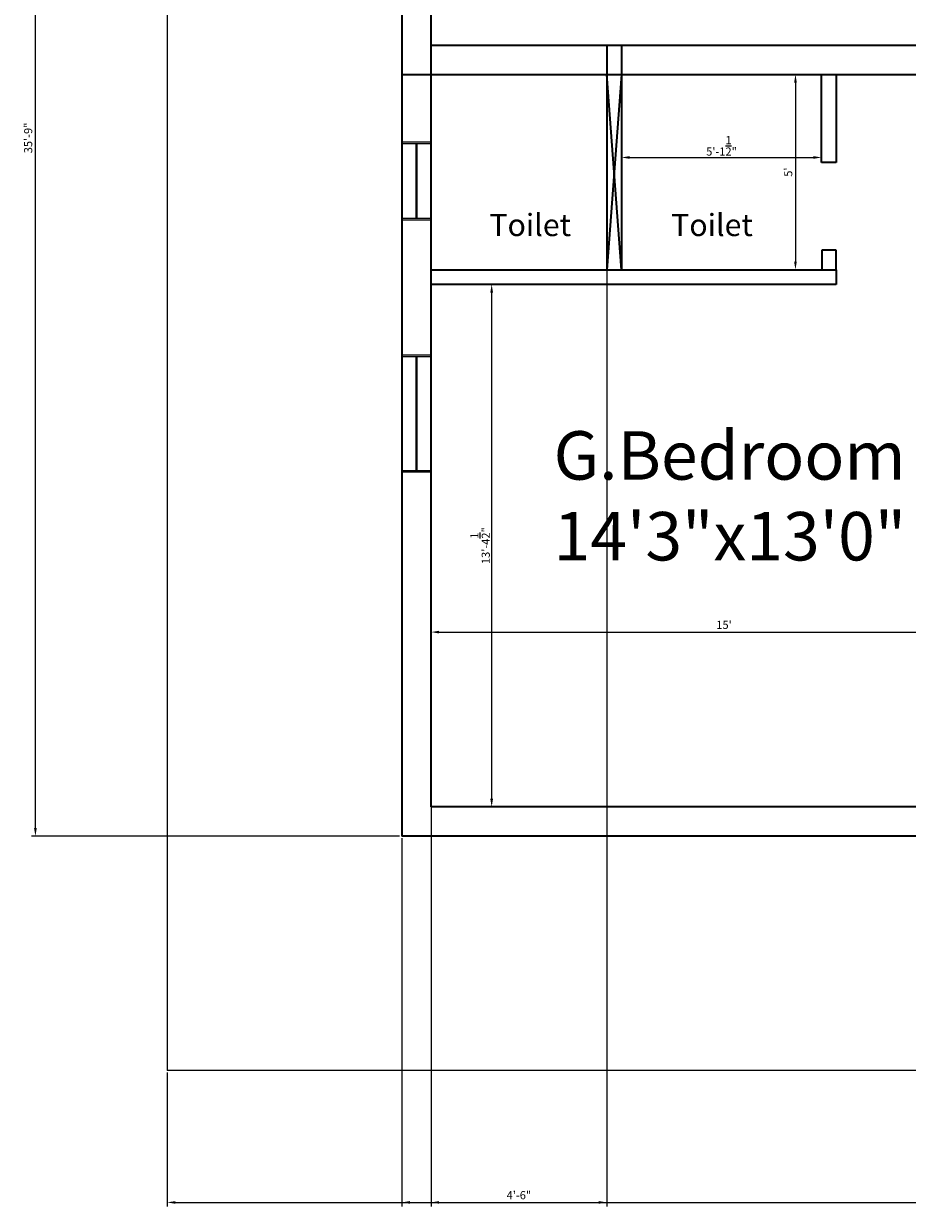
# Model space of a CAD drawing. Units: inches. Extents: x 250205121 to 250208111, y 89832590 to 89833271.
# Tile 5 of 14: x 250206174 to 250206445, y 89832600 to 89832964. Entities that reach past the tile are written whole.
import ezdxf

# ---------------------------------------------------------------- set-up
doc = ezdxf.new("R2010")
doc.units = ezdxf.units.IN
for name, color, linetype, lineweight in [('A-AREA-IDEN', 4, 'Continuous', 18), ('A-WALL', 7, 'Continuous', 35), ('C-PROP', 8, 'Continuous', 25), ('dimensions', 2, 'Continuous', 18), ('window', 4, 'Continuous', 18)]:
    doc.layers.add(name, color=color, linetype=linetype, lineweight=lineweight)
doc.styles.get("Standard").update_dxf_attribs({"font": 'arial.ttf'})
doc.dimstyles.new('ISO-25', dxfattribs={"dimtxt": 2.5, "dimasz": 2.5, "dimexe": 1.25, "dimexo": 0.625, "dimtad": 1, "dimlunit": 4, "dimtxsty": 'Standard', "dimcen": 2.5, "dimadec": 0, "dimazin": 0, "dimtfac": 1, "dimtmove": 0, "dimatfit": 3, "dimfxl": 1, "dimarcsym": 0})

# ---------------------------------------------------------------- blocks, each defined once
blk = doc.blocks.new('*D12')
at = {"layer": 'Defpoints', "color": 0, "transparency": 16777216}
for p in [(250206357.69, 89832922.83), (250206419.16, 89832922.83), (250206419.16, 89832922.83)]:
    blk.add_point(p, dxfattribs=at)
at = {"layer": 'dimensions', "color": 0, "lineweight": -2, "transparency": 16777216}
for p, q in [((250206357.69, 89832923.45), (250206357.69, 89832924.08)), ((250206360.19, 89832922.83), (250206416.66, 89832922.83)), ((250206419.16, 89832923.45), (250206419.16, 89832924.08))]:
    blk.add_line(p, q, dxfattribs=at)
at = {"layer": 'dimensions', "color": 0, "transparency": 16777216}
for points in [[(250206360.19, 89832923.24), (250206360.19, 89832922.41), (250206357.69, 89832922.83)], [(250206416.66, 89832923.24), (250206416.66, 89832922.41), (250206419.16, 89832922.83)]]:
    blk.add_solid(points, dxfattribs=at)
at = {"layer": 'dimensions', "color": 0, "transparency": 16777216, "insert": (250206388.43, 89832926.4), "char_height": 2.5, "attachment_point": 5}
blk.add_mtext('5\'-1{\\H1x;\\S1/2;}"', dxfattribs=at)
blk = doc.blocks.new('*D13')
at = {"layer": 'Defpoints', "color": 0, "transparency": 16777216}
for p in [(250206401.38, 89832948.33), (250206401.38, 89832888.33), (250206411.13, 89832888.33)]:
    blk.add_point(p, dxfattribs=at)
at = {"layer": 'dimensions', "color": 0, "lineweight": -2, "transparency": 16777216}
for p, q in [((250206402, 89832948.33), (250206412.38, 89832948.33)), ((250206411.13, 89832945.83), (250206411.13, 89832890.83)), ((250206402, 89832888.33), (250206412.38, 89832888.33))]:
    blk.add_line(p, q, dxfattribs=at)
at = {"layer": 'dimensions', "color": 0, "transparency": 16777216}
for points in [[(250206410.72, 89832945.83), (250206411.55, 89832945.83), (250206411.13, 89832948.33)], [(250206410.72, 89832890.83), (250206411.55, 89832890.83), (250206411.13, 89832888.33)]]:
    blk.add_solid(points, dxfattribs=at)
at = {"layer": 'dimensions', "color": 0, "transparency": 16777216, "insert": (250206409.24, 89832918.33), "char_height": 2.5, "attachment_point": 5, "rotation": 90}
blk.add_mtext("5'", dxfattribs=at)
blk = doc.blocks.new('*D14')
at = {"layer": 'Defpoints', "color": 0, "transparency": 16777216}
for p in [(250206479.19, 89832777.03), (250206299.19, 89832769.11), (250206479.19, 89832769.11)]:
    blk.add_point(p, dxfattribs=at)
at = {"layer": 'dimensions', "color": 0, "lineweight": -2, "transparency": 16777216}
for p, q in [((250206299.19, 89832769.73), (250206299.19, 89832778.28)), ((250206301.69, 89832777.03), (250206476.69, 89832777.03)), ((250206479.19, 89832769.73), (250206479.19, 89832778.28))]:
    blk.add_line(p, q, dxfattribs=at)
at = {"layer": 'dimensions', "color": 0, "transparency": 16777216}
for points in [[(250206301.69, 89832777.44), (250206301.69, 89832776.61), (250206299.19, 89832777.03)], [(250206476.69, 89832777.44), (250206476.69, 89832776.61), (250206479.19, 89832777.03)]]:
    blk.add_solid(points, dxfattribs=at)
at = {"layer": 'dimensions', "color": 0, "transparency": 16777216, "insert": (250206389.19, 89832778.93), "char_height": 2.5, "attachment_point": 5}
blk.add_mtext("15'", dxfattribs=at)
blk = doc.blocks.new('*D15')
at = {"layer": 'Defpoints', "color": 0, "transparency": 16777216}
for p in [(250206320.26, 89832883.83), (250206317.82, 89832723.33), (250206320.26, 89832723.33)]:
    blk.add_point(p, dxfattribs=at)
at = {"layer": 'dimensions', "color": 0, "lineweight": -2, "transparency": 16777216}
for p, q in [((250206319.63, 89832883.83), (250206316.57, 89832883.83)), ((250206317.82, 89832881.33), (250206317.82, 89832725.83)), ((250206319.63, 89832723.33), (250206316.57, 89832723.33))]:
    blk.add_line(p, q, dxfattribs=at)
at = {"layer": 'dimensions', "color": 0, "transparency": 16777216}
for points in [[(250206317.4, 89832881.33), (250206318.24, 89832881.33), (250206317.82, 89832883.83)], [(250206317.4, 89832725.83), (250206318.24, 89832725.83), (250206317.82, 89832723.33)]]:
    blk.add_solid(points, dxfattribs=at)
at = {"layer": 'dimensions', "color": 0, "transparency": 16777216, "insert": (250206314.25, 89832803.58), "char_height": 2.5, "attachment_point": 5, "rotation": 90}
blk.add_mtext('13\'-4{\\H1x;\\S1/2;}"', dxfattribs=at)
blk = doc.blocks.new('WIN-24IN')
for p, q in [((0, 0), (0, 24.08)), ((0, 24.08), (9, 24.08)), ((0, 23.58), (9, 23.58)), ((4.3, 23.58), (4.3, 0.5)), ((4.7, 23.58), (4.7, 0.5)), ((9, 24.08), (9, 0)), ((9, 0.5), (0, 0.5)), ((9, 0), (0, 0))]:
    blk.add_line(p, q)
blk = doc.blocks.new('WIN-36IN')
for p, q in [((0, 0), (0, 36.08)), ((0, 36.08), (9, 36.08)), ((0, 35.58), (9, 35.58)), ((4.3, 35.58), (4.3, 0.5)), ((4.7, 35.58), (4.7, 0.5)), ((9, 36.08), (9, 0)), ((9, 0.5), (0, 0.5)), ((9, 0), (0, 0))]:
    blk.add_line(p, q)
blk = doc.blocks.new('*D54')
at = {"layer": 'Defpoints', "color": 0, "transparency": 16777216}
for p in [(250206218.19, 89832642.33), (250207020.69, 89832642.33), (250207020.69, 89832601.83)]:
    blk.add_point(p, dxfattribs=at)
at = {"layer": 'dimensions', "color": 0, "lineweight": -2, "transparency": 16777216}
for p, q in [((250206218.19, 89832641.7), (250206218.19, 89832600.58)), ((250207020.69, 89832641.7), (250207020.69, 89832600.58)), ((250206220.69, 89832601.83), (250207018.19, 89832601.83))]:
    blk.add_line(p, q, dxfattribs=at)
at = {"layer": 'dimensions', "color": 0, "transparency": 16777216}
for points in [[(250206220.69, 89832602.24), (250206220.69, 89832601.41), (250206218.19, 89832601.83)], [(250207018.19, 89832602.24), (250207018.19, 89832601.41), (250207020.69, 89832601.83)]]:
    blk.add_solid(points, dxfattribs=at)
at = {"layer": 'dimensions', "color": 0, "transparency": 16777216, "insert": (250206619.44, 89832603.75), "char_height": 2.5, "attachment_point": 5}
blk.add_mtext('66\'-10 1/2"', dxfattribs=at)
blk = doc.blocks.new('*D59')
at = {"layer": 'Defpoints', "color": 0, "transparency": 16777216}
for p in [(250206177.69, 89833143.33), (250206290.19, 89833143.33), (250206290.19, 89832714.33)]:
    blk.add_point(p, dxfattribs=at)
at = {"layer": 'dimensions', "color": 0, "lineweight": -2, "transparency": 16777216}
for p, q in [((250206289.56, 89833143.33), (250206176.44, 89833143.33)), ((250206177.69, 89832716.83), (250206177.69, 89833140.83)), ((250206289.56, 89832714.33), (250206176.44, 89832714.33))]:
    blk.add_line(p, q, dxfattribs=at)
at = {"layer": 'dimensions', "color": 0, "transparency": 16777216}
for points in [[(250206177.27, 89833140.83), (250206178.1, 89833140.83), (250206177.69, 89833143.33)], [(250206177.27, 89832716.83), (250206178.1, 89832716.83), (250206177.69, 89832714.33)]]:
    blk.add_solid(points, dxfattribs=at)
at = {"layer": 'dimensions', "color": 0, "transparency": 16777216, "insert": (250206175.78, 89832928.83), "char_height": 2.5, "attachment_point": 5, "rotation": 90}
blk.add_mtext('35\'-9"', dxfattribs=at)
blk = doc.blocks.new('*D60')
at = {"layer": 'Defpoints', "color": 0, "transparency": 16777216}
for p in [(250206299.19, 89832957.33), (250206353.19, 89832948.33), (250206353.19, 89832601.83)]:
    blk.add_point(p, dxfattribs=at)
at = {"layer": 'dimensions', "color": 0, "lineweight": -2, "transparency": 16777216}
for p, q in [((250206299.19, 89832956.7), (250206299.19, 89832600.58)), ((250206353.19, 89832947.7), (250206353.19, 89832600.58)), ((250206301.69, 89832601.83), (250206350.69, 89832601.83))]:
    blk.add_line(p, q, dxfattribs=at)
at = {"layer": 'dimensions', "color": 0, "transparency": 16777216}
for points in [[(250206301.69, 89832602.24), (250206301.69, 89832601.41), (250206299.19, 89832601.83)], [(250206350.69, 89832602.24), (250206350.69, 89832601.41), (250206353.19, 89832601.83)]]:
    blk.add_solid(points, dxfattribs=at)
at = {"layer": 'dimensions', "color": 0, "transparency": 16777216, "insert": (250206326.19, 89832603.73), "char_height": 2.5, "attachment_point": 5}
blk.add_mtext('4\'-6"', dxfattribs=at)
blk = doc.blocks.new('*D61')
at = {"layer": 'Defpoints', "color": 0, "transparency": 16777216}
for p in [(250206290.19, 89832714.33), (250206924.69, 89832714.33), (250206924.69, 89832601.83)]:
    blk.add_point(p, dxfattribs=at)
at = {"layer": 'dimensions', "color": 0, "lineweight": -2, "transparency": 16777216}
for p, q in [((250206290.19, 89832713.7), (250206290.19, 89832600.58)), ((250206924.69, 89832713.7), (250206924.69, 89832600.58)), ((250206292.69, 89832601.83), (250206922.19, 89832601.83))]:
    blk.add_line(p, q, dxfattribs=at)
at = {"layer": 'dimensions', "color": 0, "transparency": 16777216}
for points in [[(250206292.69, 89832602.24), (250206292.69, 89832601.41), (250206290.19, 89832601.83)], [(250206922.19, 89832602.24), (250206922.19, 89832601.41), (250206924.69, 89832601.83)]]:
    blk.add_solid(points, dxfattribs=at)
at = {"layer": 'dimensions', "color": 0, "transparency": 16777216, "insert": (250206607.44, 89832603.75), "char_height": 2.5, "attachment_point": 5}
blk.add_mtext('52\'-10 1/2"', dxfattribs=at)

msp = doc.modelspace()

# ---------------------------------------------------------------- linework, layer by layer
at = {"layer": 'A-WALL'}
for p, q in [((250206290.187, 89833091.828), (250206290.187, 89832714.328)), ((250206299.187, 89833091.828), (250206299.187, 89832723.328)), ((250206299.187, 89832957.328), (250206534.687, 89832957.328)), ((250206353.187, 89832957.328), (250206353.187, 89832888.328)), ((250206357.687, 89832957.328), (250206357.687, 89832888.328)), ((250206290.187, 89832948.328), (250206534.687, 89832948.328)), ((250206357.687, 89832888.328), (250206353.187, 89832948.328)), ((250206357.687, 89832948.328), (250206353.187, 89832888.328)), ((250206419.165, 89832921.328), (250206419.165, 89832948.328)), ((250206423.665, 89832948.328), (250206423.665, 89832921.328)), ((250206423.665, 89832921.328), (250206419.165, 89832921.328)), ((250206423.687, 89832894.328), (250206419.187, 89832894.328)), ((250206419.187, 89832894.328), (250206419.187, 89832888.328)), ((250206423.687, 89832888.328), (250206423.687, 89832894.328)), ((250206299.187, 89832888.328), (250206423.687, 89832888.328)), ((250206423.687, 89832888.328), (250206423.687, 89832883.828)), ((250206423.687, 89832883.828), (250206299.187, 89832883.828)), ((250206840.687, 89832723.328), (250206299.187, 89832723.328)), ((250206392.714, 89832714.328), (250206290.187, 89832714.328)), ((250206840.687, 89832714.328), (250206307.687, 89832714.328))]:
    msp.add_line(p, q, dxfattribs=at)
at = {"layer": 'C-PROP'}
for p in [(250206218.187, 89833215.328), (250206543.687, 89832642.328)]:
    msp.add_line(p, (250206218.187, 89832642.328), dxfattribs=at)

# ---------------------------------------------------------------- block references
at = {"layer": 'window'}
for name, p in [('WIN-24IN', (250206290.187, 89832903.549)), ('WIN-36IN', (250206290.187, 89832826.107))]:
    msp.add_blockref(name, p, dxfattribs=at)

# ---------------------------------------------------------------- texts
at = {"layer": 'A-AREA-IDEN', "attachment_point": 1}
for s, width, gutter_width, insert, char_height in [('Toilet', 7.46996, 34.11, (250206317.121, 89832905.502), 6.8219), ('Toilet', 7.46996, 34.11, (250206372.954, 89832905.502), 6.8219), ('G.Bedroom\\P14\'3"x13\'0"', 23.63705, 74.43, (250206336.849, 89832838.737), 14.88606)]:
    msp.add_mtext_dynamic_manual_height_columns(s, width=width, gutter_width=gutter_width, heights=[0], dxfattribs=dict(at, insert=insert, char_height=char_height))

# ---------------------------------------------------------------- dimensions: what is measured, and where the dimension line sits
at = {"layer": 'dimensions'}
for base, p1, p2, override, picture, middle in [((250206177.687, 89833143.328), (250206290.187, 89832714.328), (250206290.187, 89833143.328), {"dimdec": 1, "dimlfac": 1, "dimrnd": 0, "dimzin": 1, "dimdsep": 46, "dimlunit": 4, "dimfrac": 2}, '*D59', (250206175.785, 89832928.828)), ((250206411.134, 89832888.328), (250206401.378, 89832948.328), (250206401.378, 89832888.328), {"dimclrd": 0, "dimclre": 0, "dimclrt": 0}, '*D13', (250206409.238, 89832918.328)), ((250206317.819, 89832723.328), (250206320.258, 89832883.828), (250206320.258, 89832723.328), {"dimclrd": 0, "dimclre": 0, "dimclrt": 0}, '*D15', (250206314.245, 89832803.578))]:
    dim = msp.add_linear_dim(base=base, p1=p1, p2=p2, angle=90, dimstyle='ISO-25', override=override, dxfattribs=at)
    dim.commit()
    dim.dimension.update_dxf_attribs({"geometry": picture, "text_midpoint": middle})
for base, p1, p2, override, picture, middle in [((250206353.187, 89832601.828), (250206299.187, 89832957.328), (250206353.187, 89832948.328), {"dimdec": 1, "dimlfac": 1, "dimrnd": 0, "dimzin": 1, "dimdsep": 46, "dimlunit": 4, "dimfrac": 2}, '*D60', (250206326.187, 89832603.729)), ((250206419.165, 89832922.828), (250206357.687, 89832922.828), (250206419.165, 89832922.828), {"dimclrd": 0, "dimclre": 0, "dimclrt": 0}, '*D12', (250206388.426, 89832926.401)), ((250206479.187, 89832777.026), (250206299.187, 89832769.105), (250206479.187, 89832769.105), {"dimclrd": 0, "dimclre": 0, "dimclrt": 0}, '*D14', (250206389.187, 89832778.928)), ((250206924.687, 89832601.828), (250206290.187, 89832714.328), (250206924.687, 89832714.328), {"dimdec": 1, "dimlfac": 1, "dimrnd": 0, "dimzin": 1, "dimdsep": 46, "dimlunit": 4, "dimfrac": 2}, '*D61', (250206607.437, 89832603.746)), ((250207020.687, 89832601.828), (250206218.187, 89832642.328), (250207020.687, 89832642.328), {"dimdec": 1, "dimlfac": 1, "dimrnd": 0, "dimzin": 1, "dimdsep": 46, "dimlunit": 4, "dimfrac": 2}, '*D54', (250206619.437, 89832603.746))]:
    dim = msp.add_linear_dim(base=base, p1=p1, p2=p2, dimstyle='ISO-25', override=override, dxfattribs=at)
    dim.commit()
    dim.dimension.update_dxf_attribs({"geometry": picture, "text_midpoint": middle})

doc.saveas('drawing.dxf')
